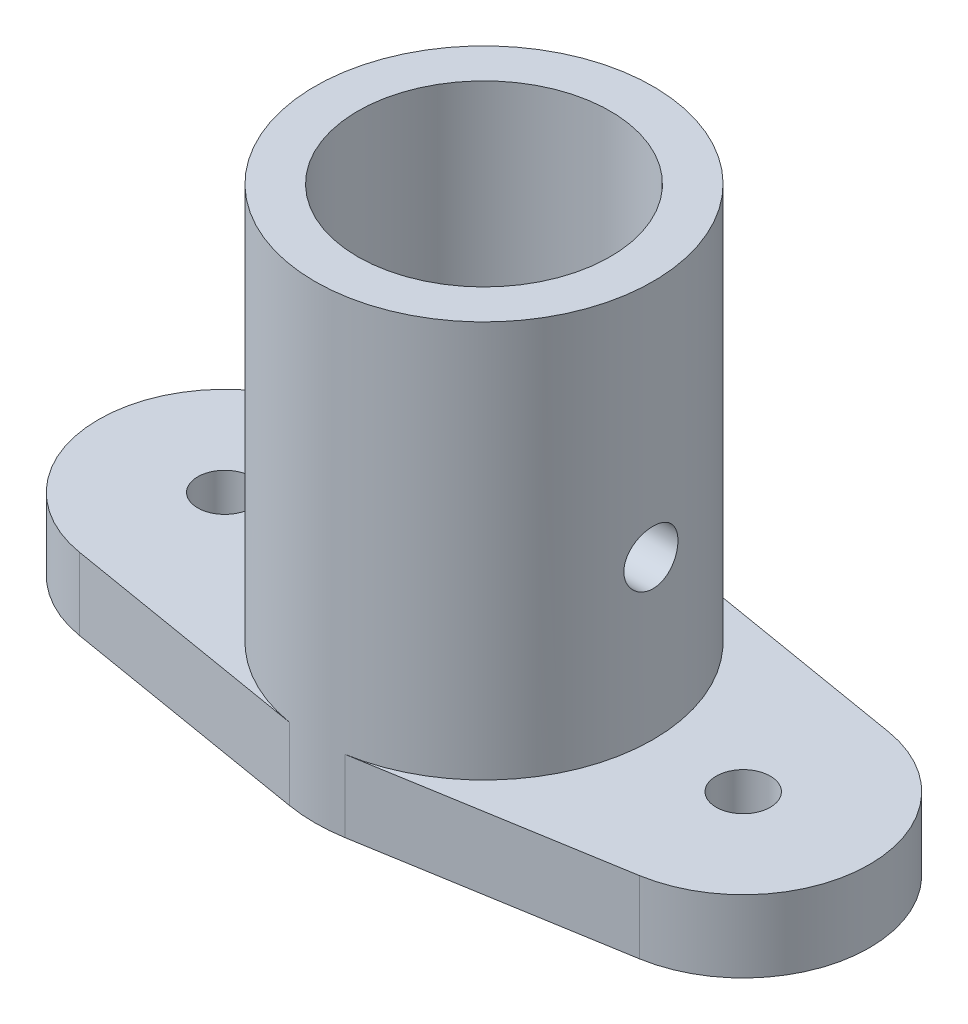
SolidWorks part; units mm, degrees
material "Plain Carbon Steel"
ref_plane "Front Plane" through (0, 0, 0) normal (0, 0, 1) x (1, 0, 0)
ref_plane "Top Plane" through (0, 0, 0) normal (0, 1, 0) x (1, 0, 0)
ref_plane "Right Plane" through (0, 0, 0) normal (1, 0, 0) x (0, 0, -1)
sketch "Base Flange Sketch" plane through (0, 0, 0) normal (0, 1, 0) x (1, 0, 0)
  line L0 (0, 0) -> (0, 37.8581) construction
  line L1 (-62.1261, -27.6152) -> (-6.1957, -36.9846)
  line L2 (6.1957, -36.9846) -> (62.1261, -27.6152)
  line L3 (62.1261, 27.6152) -> (6.1957, 36.9846)
  line L4 (-6.1957, 36.9846) -> (-62.1261, 27.6152)
  arc A0 (-6.1957, -36.9846) -> (6.1957, -36.9846) centre (0, 0) ccw
  circle A1 centre (-57.5, 0) radius 6
  arc A2 (-62.1261, 27.6152) -> (-62.1261, -27.6152) centre (-57.5, 0) ccw
  circle A3 centre (57.5, 0) radius 6
  arc A4 (62.1261, -27.6152) -> (62.1261, 27.6152) centre (57.5, 0) ccw
  arc A5 (6.1957, 36.9846) -> (-6.1957, 36.9846) centre (0, 0) ccw
  dimension "D1" = 12
  dimension "D2" = 28
  dimension "D3" = 75
  dimension "D4" = 115
extrude "Base Flange" add sketch "Base Flange Sketch" along normal mid plane 16
sketch "Tube Sketch" plane through (0, 8, 0) normal (0, 1, 0) x (1, 0, 0)
  circle A0 centre (0, 0) radius 37.5
  dimension "D1" = 75
extrude "Tube Ø75" add sketch "Tube Sketch" along normal blind 88
sketch "Bore Sketch" plane through (0, 96, 0) normal (0, 1, 0) x (1, 0, 0)
  circle A0 centre (0, 0) radius 28
  dimension "D1" = 56
extrude "Bore Ø56" cut sketch "Bore Sketch" against normal blind 76
sketch "Spigot Sketch" plane through (0, -8, 0) normal (0, -1, 0) x (1, 0, 0)
  circle A0 centre (0, 0) radius 19
  dimension "D1" = 38
extrude "Spigot Ø38" add sketch "Spigot Sketch" along normal blind 6
sketch "Spigot Hole Sketch" plane through (0, -14, 0) normal (0, -1, 0) x (1, 0, 0)
  circle A0 centre (0, 0) radius 11
  dimension "D1" = 22
extrude "Spigot Hole Ø22" cut sketch "Spigot Hole Sketch" against normal blind 22
sketch "Bore Step Sketch" plane through (0, 20, 0) normal (0, 1, 0) x (1, 0, 0)
  circle A0 centre (0, 0) radius 22.5
  dimension "D1" = 45
extrude "Bore Step Ø45" cut sketch "Bore Step Sketch" against normal blind 12
sketch "Cross Hole Sketch" plane through (0, 0, 0) normal (1, 0, 0) x (0, 0, -1)
  line L0 (28, 96) -> (-28, 96) construction
  circle A0 centre (0, 43) radius 6
  dimension "D1" = 12
  dimension "D2" = 53
extrude "Cross Hole Ø12" cut sketch "Cross Hole Sketch" against normal through all both and the other way through all
